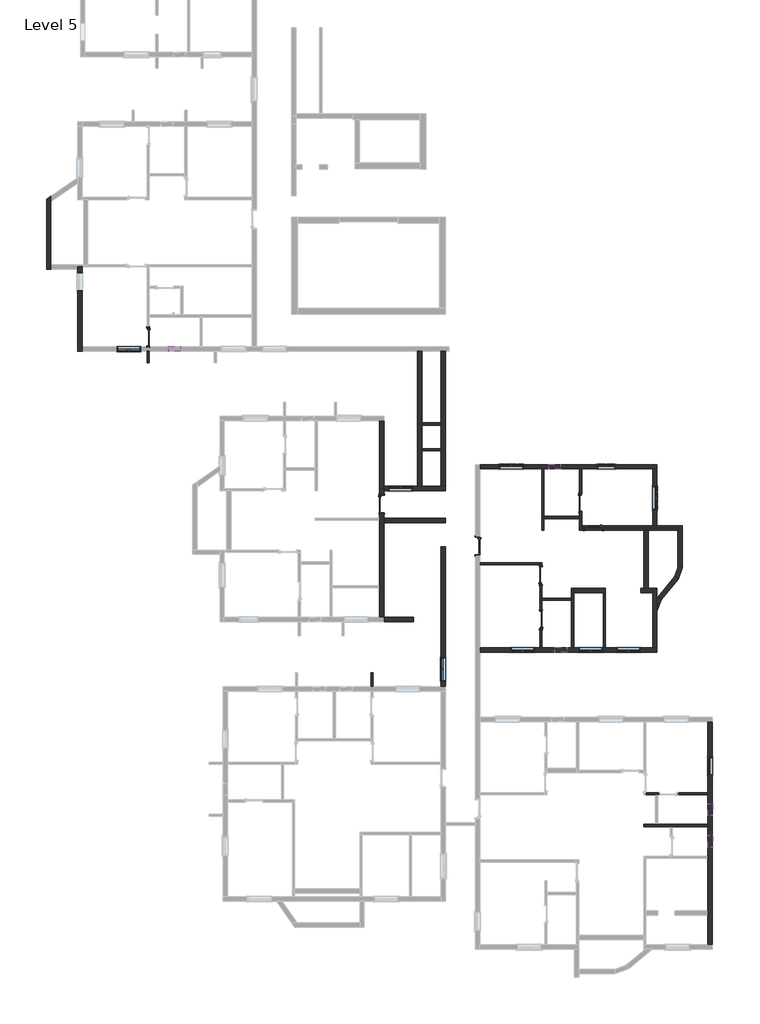
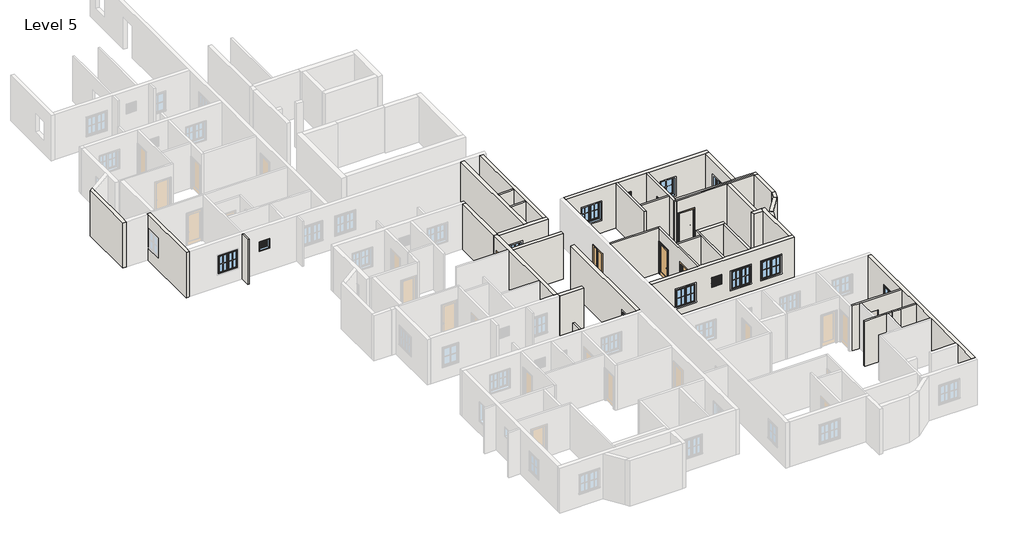
# One storey, part 3 of 7: 39 walls, 15 windows, 7 doors.
# Revit data of these elements (continued)
# Element 52 (IfcWindow, "Window-Casement-Double : 4' x 4'") (continued)
#   Interior Wall Closure = 0' - 2 1/4"
#   Frame Extension = 0' - 0 1/4"
#   Exterior Wall Closure = 0' - 1 1/4"
#   Interior Trim Visibility = yes
#   Exterior Trim Visibility = yes
#   Phase Created = New Construction
#   Materials on its faces: "Wood - Stained", "Glass", "Clad - White"
# Element 53 (IfcWindow, "Window-Casement-Double : 4' x 4'")
#   Mark = "110"
#   Window Inset = 0' - 0"
#   Interior Wall Closure = 0' - 2 1/4"
#   Frame Extension = 0' - 0 1/4"
#   Exterior Wall Closure = 0' - 1 1/4"
#   Interior Trim Visibility = yes
#   Exterior Trim Visibility = yes
#   Phase Created = New Construction
#   Materials on its faces: "Wood - Stained", "Glass", "Clad - White"
# Element 54 (IfcWindow, "Window-Casement-Double : 4' x 4'")
#   Mark = "121"
#   Window Inset = 0' - 0"
#   Interior Wall Closure = 0' - 2 1/4"
#   Frame Extension = 0' - 0 1/4"
#   Exterior Wall Closure = 0' - 1 1/4"
#   Interior Trim Visibility = yes
#   Exterior Trim Visibility = yes
#   Phase Created = New Construction
#   Materials on its faces: "Wood - Stained", "Glass", "Clad - White"
# Element 55 (IfcWindow, "Window-Casement-Double : 4' x 4'")
#   Mark = "124"
#   Window Inset = 0' - 0"
#   Interior Wall Closure = 0' - 2 1/4"
#   Frame Extension = 0' - 0 1/4"
#   Exterior Wall Closure = 0' - 1 1/4"
#   Interior Trim Visibility = yes
#   Exterior Trim Visibility = yes
#   Phase Created = New Construction
#   Materials on its faces: "Wood - Stained", "Glass", "Clad - White"
# Element 56 (IfcWindow, "Window-Casement-Double : 4' x 4'")
#   Mark = "129"
#   Window Inset = 0' - 0"
#   Interior Wall Closure = 0' - 2 1/4"
#   Frame Extension = 0' - 0 1/4"
#   Exterior Wall Closure = 0' - 1 1/4"
#   Interior Trim Visibility = yes
#   Exterior Trim Visibility = yes
#   Phase Created = New Construction
#   Materials on its faces: "Wood - Stained", "Glass", "Clad - White"
# Element 57 (IfcWindow, "Window-Louvers : 24\" x 24\"")
#   Mark = "72"
#   Blade Width = 1' - 10 1/2"
#   Phase Created = New Construction
#   Materials on its faces: "Birch"
# Element 58 (IfcWindow, "Window-Louvers : 24\" x 24\"")
#   Mark = "75"
#   Blade Width = 1' - 10 1/2"
#   Phase Created = New Construction
#   Materials on its faces: "Birch"
# Element 59 (IfcWindow, "Window-Louvers : 24\" x 24\"")
#   Mark = "76"
#   Blade Width = 1' - 10 1/2"
#   Phase Created = New Construction
#   Materials on its faces: "Birch"
# Element 60 (IfcWindow, "Window-Louvers : 24\" x 24\"")
#   Mark = "81"
#   Blade Width = 1' - 10 1/2"
#   Phase Created = New Construction
#   Materials on its faces: "Birch"
# Element 61 (IfcWindow, "Window-Louvers : 24\" x 24\"")
#   Mark = "82"
#   Blade Width = 1' - 10 1/2"
#   Phase Created = New Construction
#   Materials on its faces: "Birch"
# Materials
#   "Cherry": class "Wood", colour RGB 226 177 128, transparency 0, Description = "Prunus Serotina", Cost = 0
#   "Aluminum": class "Metal", colour RGB 247 247 247, transparency 0, Description = "Aluminum 6061", Cost = 0
#   "Wood - Stained": class "Wood", colour RGB 224 178 126, transparency 0, Cost = 0
#   "Glass": class "Glass", colour RGB 0 128 192, transparency 0.75, Description = "Soda Lime Glass", Cost = 0
#   "Clad - White": class "Wood", colour RGB 242 242 238, transparency 0, Cost = 0
#   "Birch": class "Wood", colour RGB 224 178 126, transparency 0, Description = "Betula Alleghaniensis", Cost = 0
#   "Default Wall": colour RGB 128 128 128, transparency 0, Cost = 0
